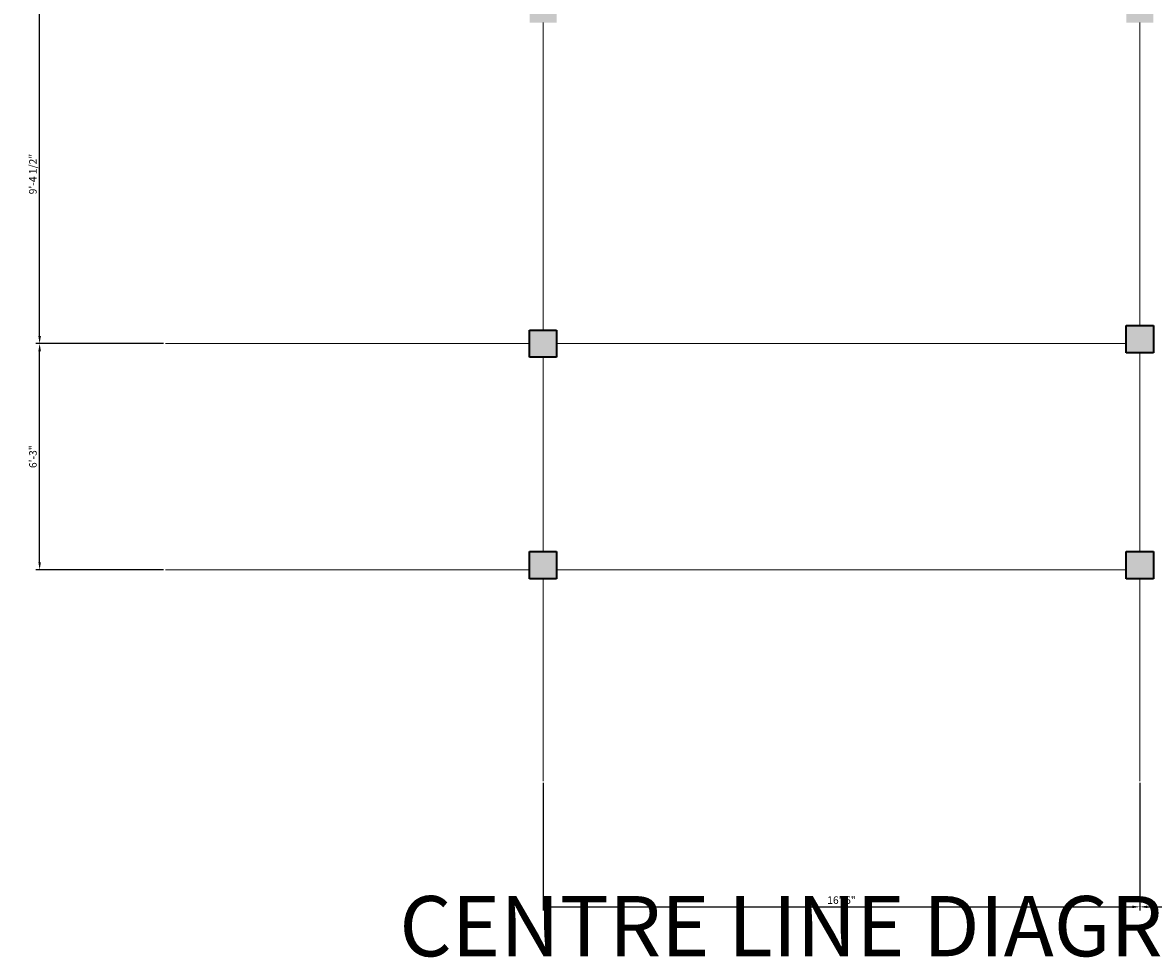
# Model space of a CAD drawing. Units: inches. Extents: x 6038 to 7543, y 3772 to 5131.
# Tile 10 of 14: x 6806 to 7182, y 4237 to 4547. Entities that reach past the tile are written whole.
import ezdxf

# ---------------------------------------------------------------- set-up
doc = ezdxf.new("R2010")
doc.units = ezdxf.units.IN
for name, color, linetype, lineweight in [('A-ANNO-DIMS', 4, 'Continuous', 18), ('A-ANNO-TITL', 3, 'Continuous', 30), ('S-COLS', 7, 'Continuous', 35), ('S-COLS-PATT', 9, 'Continuous', 13), ('S-GRID', 6, 'Continuous', 13)]:
    doc.layers.add(name, color=color, linetype=linetype, lineweight=lineweight)
doc.styles.get("Standard").update_dxf_attribs({"font": 'arial.ttf'})
doc.dimstyles.new('ISO-25', dxfattribs={"dimtxt": 2.5, "dimasz": 2.5, "dimexe": 1.25, "dimexo": 0.625, "dimtad": 1, "dimdec": 0, "dimlunit": 3, "dimtxsty": 'Standard', "dimcen": 2.5, "dimadec": 0, "dimazin": 0, "dimtfac": 1, "dimtdec": 0, "dimtmove": 0, "dimatfit": 3, "dimfxl": 1, "dimarcsym": 0})

# ---------------------------------------------------------------- blocks, each defined once
blk = doc.blocks.new('COL-9X9')
for p, q in [((0, 9), (9, 9)), ((0, 0), (0, 9)), ((9, 9), (9, 0)), ((9, 0), (0, 0))]:
    blk.add_line(p, q)
blk = doc.blocks.new('*D85')
at = {"layer": 'A-ANNO-DIMS', "color": 0, "lineweight": -2, "transparency": 16777216}
for p, q in [((6979.09, 4294.9), (6979.09, 4252.53)), ((7177.09, 4294.9), (7177.09, 4252.53)), ((6981.59, 4253.78), (7174.59, 4253.78))]:
    blk.add_line(p, q, dxfattribs=at)
at = {"layer": 'A-ANNO-DIMS', "color": 0, "transparency": 16777216}
for points in [[(6981.59, 4254.2), (6981.59, 4253.36), (6979.09, 4253.78)], [(7174.59, 4254.2), (7174.59, 4253.36), (7177.09, 4253.78)]]:
    blk.add_solid(points, dxfattribs=at)
at = {"layer": 'Defpoints', "color": 0, "transparency": 16777216}
for p in [(6979.09, 4295.53), (7177.09, 4295.53), (7177.09, 4253.78)]:
    blk.add_point(p, dxfattribs=at)
at = {"layer": 'A-ANNO-DIMS', "color": 0, "transparency": 16777216, "insert": (7078.09, 4255.68), "char_height": 2.5, "attachment_point": 5}
blk.add_mtext('16\'-6"', dxfattribs=at)
blk = doc.blocks.new('*D86')
at = {"layer": 'A-ANNO-DIMS', "color": 0, "lineweight": -2, "transparency": 16777216}
for p, q in [((7177.09, 4294.9), (7177.09, 4252.53)), ((7330.09, 4294.9), (7330.09, 4252.53)), ((7179.59, 4253.78), (7327.59, 4253.78))]:
    blk.add_line(p, q, dxfattribs=at)
at = {"layer": 'A-ANNO-DIMS', "color": 0, "transparency": 16777216}
for points in [[(7179.59, 4254.2), (7179.59, 4253.36), (7177.09, 4253.78)], [(7327.59, 4254.2), (7327.59, 4253.36), (7330.09, 4253.78)]]:
    blk.add_solid(points, dxfattribs=at)
at = {"layer": 'Defpoints', "color": 0, "transparency": 16777216}
for p in [(7177.09, 4295.53), (7330.09, 4295.53), (7330.09, 4253.78)]:
    blk.add_point(p, dxfattribs=at)
at = {"layer": 'A-ANNO-DIMS', "color": 0, "transparency": 16777216, "insert": (7253.59, 4255.68), "char_height": 2.5, "attachment_point": 5}
blk.add_mtext('12\'-9"', dxfattribs=at)
blk = doc.blocks.new('*D87')
at = {"layer": 'A-ANNO-DIMS', "color": 0, "lineweight": -2, "transparency": 16777216}
for p, q in [((6853.17, 4440.62), (6810.8, 4440.62)), ((6812.05, 4368.12), (6812.05, 4438.12)), ((6853.17, 4365.62), (6810.8, 4365.62))]:
    blk.add_line(p, q, dxfattribs=at)
at = {"layer": 'A-ANNO-DIMS', "color": 0, "transparency": 16777216}
for points in [[(6811.63, 4438.12), (6812.47, 4438.12), (6812.05, 4440.62)], [(6811.63, 4368.12), (6812.47, 4368.12), (6812.05, 4365.62)]]:
    blk.add_solid(points, dxfattribs=at)
at = {"layer": 'Defpoints', "color": 0, "transparency": 16777216}
for p in [(6812.05, 4440.62), (6853.8, 4440.62), (6853.8, 4365.62)]:
    blk.add_point(p, dxfattribs=at)
at = {"layer": 'A-ANNO-DIMS', "color": 0, "transparency": 16777216, "insert": (6810.15, 4403.12), "char_height": 2.5, "attachment_point": 5, "rotation": 90}
blk.add_mtext('6\'-3"', dxfattribs=at)
blk = doc.blocks.new('*D88')
at = {"layer": 'A-ANNO-DIMS', "color": 0, "lineweight": -2, "transparency": 16777216}
for p, q in [((6853.17, 4553.12), (6810.8, 4553.12)), ((6812.05, 4443.12), (6812.05, 4550.62)), ((6853.17, 4440.62), (6810.8, 4440.62))]:
    blk.add_line(p, q, dxfattribs=at)
at = {"layer": 'A-ANNO-DIMS', "color": 0, "transparency": 16777216}
for points in [[(6811.63, 4550.62), (6812.47, 4550.62), (6812.05, 4553.12)], [(6811.63, 4443.12), (6812.47, 4443.12), (6812.05, 4440.62)]]:
    blk.add_solid(points, dxfattribs=at)
at = {"layer": 'Defpoints', "color": 0, "transparency": 16777216}
for p in [(6812.05, 4553.12), (6853.8, 4553.12), (6853.8, 4440.62)]:
    blk.add_point(p, dxfattribs=at)
at = {"layer": 'A-ANNO-DIMS', "color": 0, "transparency": 16777216, "insert": (6810.13, 4496.87), "char_height": 2.5, "attachment_point": 5, "rotation": 90}
blk.add_mtext('9\'-4 1/2"', dxfattribs=at)

msp = doc.modelspace()

# ---------------------------------------------------------------- hatches: boundary and pattern name
at = {"layer": 'S-COLS-PATT'}
h = msp.add_hatch(color=256, dxfattribs=at)
h.dxf.hatch_style = 1
h.paths.add_polyline_path([(7325.59, 4944.62), (7334.59, 4944.62), (7334.59, 4956.62), (7325.59, 4956.62)])
h.paths.add_polyline_path([(7334.59, 4746.62), (7334.59, 4758.62), (7325.59, 4758.62), (7325.59, 4746.62)])
h.paths.add_polyline_path([(7181.59, 4758.62), (7172.59, 4758.62), (7172.59, 4746.62), (7181.59, 4746.62)])
h.paths.add_polyline_path([(6983.59, 4758.62), (6974.59, 4758.62), (6974.59, 4746.62), (6983.59, 4746.62)])
h.paths.add_polyline_path([(6983.59, 4559.12), (6974.59, 4559.12), (6974.59, 4547.12), (6983.59, 4547.12)])
h.paths.add_polyline_path([(7181.59, 4559.12), (7172.59, 4559.12), (7172.59, 4547.12), (7181.59, 4547.12)])
h.paths.add_polyline_path([(7334.59, 4559.12), (7325.59, 4559.12), (7325.59, 4547.12), (7334.59, 4547.12)])
h = msp.add_hatch(color=256, dxfattribs=at)
h.dxf.hatch_style = 1
h.paths.add_polyline_path([(6974.59, 4884.62), (6983.59, 4884.62), (6983.59, 4893.62), (6974.59, 4893.62)])
h.paths.add_polyline_path([(7181.59, 4893.62), (7172.59, 4893.62), (7172.59, 4884.62), (7181.59, 4884.62)])
h.paths.add_polyline_path([(6983.59, 4436.12), (6983.59, 4445.12), (6974.59, 4445.12), (6974.59, 4436.12)])
h.paths.add_polyline_path([(7181.59, 4446.62), (7172.59, 4446.62), (7172.59, 4437.62), (7181.59, 4437.62)])
h.paths.add_polyline_path([(7325.59, 4436.12), (7334.59, 4436.12), (7334.59, 4445.12), (7325.59, 4445.12)])
h.paths.add_polyline_path([(7334.59, 4371.62), (7325.59, 4371.62), (7325.59, 4362.62), (7334.59, 4362.62)])
h.paths.add_polyline_path([(7181.59, 4362.62), (7181.59, 4371.62), (7172.59, 4371.62), (7172.59, 4362.62)])
h.paths.add_polyline_path([(6974.59, 4362.62), (6983.59, 4362.62), (6983.59, 4371.62), (6974.59, 4371.62)])

# ---------------------------------------------------------------- linework, layer by layer
at = {"layer": 'S-GRID'}
for p, q in [((6979.09, 4547.12), (6979.09, 4445.12)), ((7177.09, 4547.12), (7177.09, 4446.62)), ((6974.59, 4440.62), (6853.8, 4440.62)), ((7172.59, 4440.62), (6983.59, 4440.62)), ((6979.09, 4436.12), (6979.09, 4371.62)), ((7177.09, 4437.62), (7177.09, 4371.62)), ((6974.59, 4365.62), (6853.8, 4365.62)), ((7172.59, 4365.62), (6983.59, 4365.62)), ((6979.09, 4362.62), (6979.09, 4295.53)), ((7177.09, 4362.62), (7177.09, 4295.53))]:
    msp.add_line(p, q, dxfattribs=at)

# ---------------------------------------------------------------- block references
at = {"layer": 'S-COLS'}
for p in [(7172.59, 4437.62), (6974.59, 4436.12), (6974.59, 4362.62), (7172.59, 4362.62)]:
    msp.add_blockref('COL-9X9', p, dxfattribs=at)

# ---------------------------------------------------------------- texts
at = {"layer": 'A-ANNO-TITL', "insert": (6931.39, 4257.37), "char_height": 20, "attachment_point": 1}
msp.add_mtext_dynamic_manual_height_columns('CENTRE LINE DIAGRAM', width=549.9641, gutter_width=12.5, heights=[0], dxfattribs=at)

# ---------------------------------------------------------------- dimensions: what is measured, and where the dimension line sits
at = {"layer": 'A-ANNO-DIMS'}
for base, p1, p2, picture, middle in [((6812.05, 4553.12), (6853.8, 4440.62), (6853.8, 4553.12), '*D88', (6810.13, 4496.87)), ((6812.05, 4440.62), (6853.8, 4365.62), (6853.8, 4440.62), '*D87', (6810.15, 4403.12))]:
    dim = msp.add_linear_dim(base=base, p1=p1, p2=p2, angle=90, dimstyle='ISO-25', override={"dimdec": 1, "dimlfac": 1, "dimrnd": 0, "dimzin": 1, "dimdsep": 46, "dimlunit": 4, "dimfrac": 2}, dxfattribs=at)
    dim.commit()
    dim.dimension.update_dxf_attribs({"geometry": picture, "text_midpoint": middle})
for base, p1, p2, picture, middle in [((7177.09, 4253.78), (6979.09, 4295.53), (7177.09, 4295.53), '*D85', (7078.09, 4255.68)), ((7330.09, 4253.78), (7177.09, 4295.53), (7330.09, 4295.53), '*D86', (7253.59, 4255.68))]:
    dim = msp.add_linear_dim(base=base, p1=p1, p2=p2, dimstyle='ISO-25', override={"dimdec": 1, "dimlfac": 1, "dimrnd": 0, "dimzin": 1, "dimdsep": 46, "dimlunit": 4, "dimfrac": 2}, dxfattribs=at)
    dim.commit()
    dim.dimension.update_dxf_attribs({"geometry": picture, "text_midpoint": middle})

doc.saveas('drawing.dxf')
